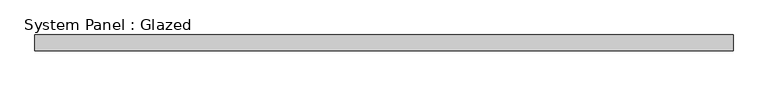
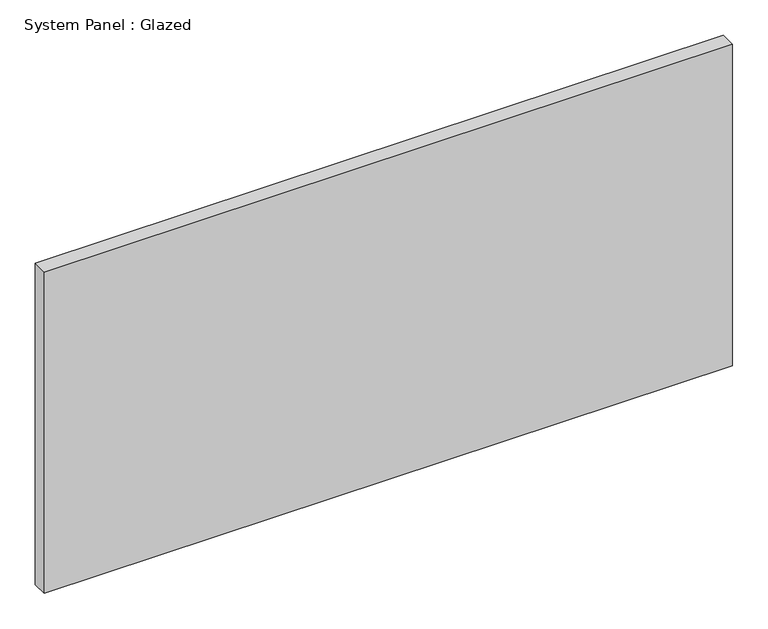
"""IFC4 building model written with IfcOpenShell, lengths in millimetres: plate geometry, System Panel : Glazed."""

from ifc_helpers import new_model, si_unit, origin, origin_with_axes, place, context, project, spatial, polyline, outline, extrude, source, transform, mapped, element, save


def system_panel_glazed_d1e8daba(model_context):
    return source(origin(), model_context, "Body", "SweptSolid", [
        extrude(outline(polyline([(561.975, 19.05), (-561.975, 19.05), (-561.975, 44.45), (561.975, 44.45), (561.975, 19.05)])), origin_with_axes(), (0.0, 0.0, 1.0), 554.5666667),
    ])


if __name__ == "__main__":
    model = new_model("IFC4")
    model_context = context("Model", 3, world=origin())
    ifc_project = project(units=[si_unit("LENGTHUNIT", "METRE", prefix="MILLI")], contexts=[model_context])
    site = spatial("IfcSite", under=ifc_project)
    building = spatial("IfcBuilding", under=site)
    placement = place(None, origin())
    system_panel_glazed_shape = system_panel_glazed_d1e8daba(model_context)
    element("IfcPlate", 1, ObjectType="System Panel : Glazed", at=placement, inside=building, context=model_context, shape_type="MappedRepresentation", body=[
        mapped(system_panel_glazed_shape, transform((0.0, 0.0, 0.0), x_axis=(1.0, 0.0, 0.0), y_axis=(0.0, 1.0, 0.0), z_axis=(0.0, 0.0, 1.0))),
    ])
    save(model, "model.ifc")

# Revit data of these elements
# Type "System Panel : Glazed"
#   Construction Type Id = "GSP4R"
#   Analytic Construction = "1/8 in Pilkington single glazing"
#   Visual Light Transmittance = 0.9
#   Solar Heat Gain Coefficient = 0.86
#   Heat Transfer Coefficient (U) = 1.18115 BTU/(h·ft²·°F)
#   Define Thermal Properties by = 1
# Element 1 (IfcPlate, "System Panel : Glazed")
#   Materials on its faces: "Glass"
# Materials
#   "Glass": class "Glass", colour RGB 0 128 192, transparency 0.75, Description = "Soda Lime Glass", Cost = 0
